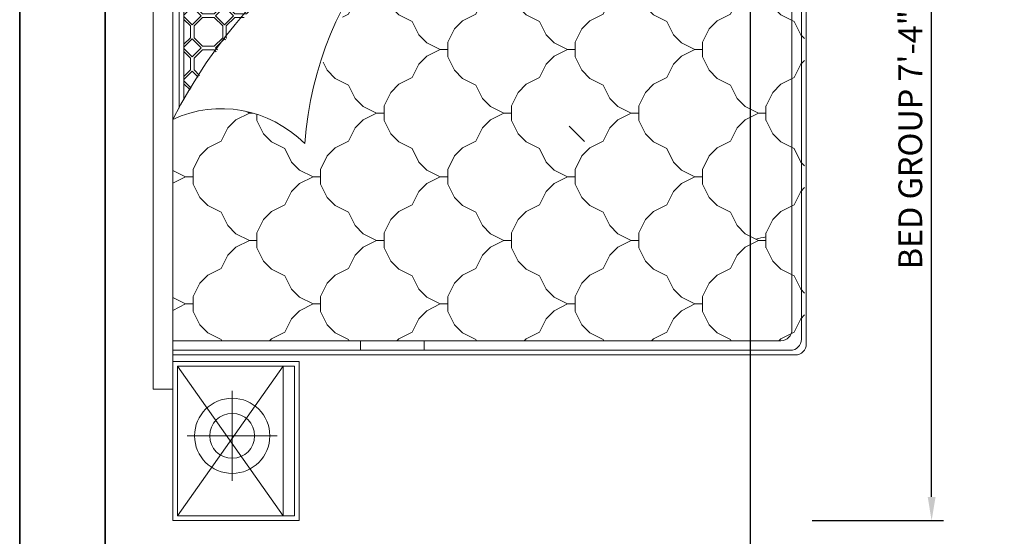
# Model space of a CAD drawing. Units: inches. Extents: x 1624 to 3956, y 1589 to 5028.
# Tile 12 of 16: x 1943 to 2046, y 2317 to 2372. Entities that reach past the tile are written whole.
import ezdxf

# ---------------------------------------------------------------- set-up
doc = ezdxf.new("R2010")
doc.units = ezdxf.units.IN
for name, color, linetype, lineweight in [('A-ANNO-DIMS', 2, 'Continuous', 13), ('A-FURN', 8, 'Continuous', 18), ('A-WALL', 7, 'Continuous', 35)]:
    doc.layers.add(name, color=color, linetype=linetype, lineweight=lineweight)
doc.styles.get("Standard").update_dxf_attribs({"font": 'arial.ttf'})
doc.dimstyles.new('Copy of ISO-25', dxfattribs={"dimtxt": 2.5, "dimasz": 2.5, "dimexe": 1.25, "dimexo": 0.625, "dimtad": 1, "dimdec": 1, "dimlunit": 4, "dimtxsty": 'Standard', "dimcen": 2.5, "dimadec": 0, "dimazin": 0, "dimtfac": 1, "dimtdec": 1, "dimtmove": 0, "dimatfit": 3, "dimfxl": 1, "dimarcsym": 0})

# ---------------------------------------------------------------- blocks, each defined once
blk = doc.blocks.new('A$C029D5C69')
for p, q in [((0.4164, 2.0693), (0.4164, 2.0066)), ((2.2315, 2.0693), (0.4164, 2.0693)), ((2.2315, 2.0066), (2.2315, 2.0693)), ((0, 1.606), (0, 2.0066)), ((0, 2.0066), (0.505, 2.0066)), ((0.4164, 2.0066), (2.2315, 2.0066)), ((0.505, 2.0066), (0.505, 1.606)), ((0.5252, 0.0351), (0.5252, 2.0066)), ((0.5403, 0.0502), (0.5403, 2.0066)), ((0.5706, 0.0805), (0.5706, 2.0066)), ((0.6869, 1.966), (0.6666, 2.0066)), ((0.7072, 2.0066), (0.6869, 1.966)), ((1.0902, 1.966), (1.0699, 2.0066)), ((1.1106, 2.0066), (1.0902, 1.966)), ((2.1114, 2.0087), (2.1114, 0.0351)), ((2.6479, 2.0066), (2.1429, 2.0066)), ((2.1429, 2.0066), (2.1429, 1.606)), ((2.6479, 1.606), (2.6479, 2.0066)), ((0.0151, 1.6211), (0.0151, 1.9915)), ((0.0151, 1.9915), (0.4899, 1.9915)), ((0.4899, 1.9915), (0.4899, 1.6211)), ((0.6869, 1.9425), (0.6869, 1.966)), ((0.6869, 1.9425), (0.6869, 1.966)), ((1.0902, 1.9425), (1.0902, 1.966)), ((1.0902, 1.9425), (1.0902, 1.966)), ((1.8954, 1.9865), (1.3081, 1.9865)), ((1.8954, 1.9713), (1.3339, 1.9713)), ((1.3849, 1.9713), (1.3656, 1.952)), ((1.3945, 1.9713), (1.3714, 1.9483)), ((1.4249, 1.945), (1.3986, 1.9713)), ((1.4288, 1.9507), (1.4081, 1.9713)), ((1.487, 1.9713), (1.4664, 1.9507)), ((1.4966, 1.9713), (1.4703, 1.945)), ((1.527, 1.945), (1.5007, 1.9713)), ((1.5309, 1.9507), (1.5102, 1.9713)), ((1.5891, 1.9713), (1.5685, 1.9507)), ((1.5987, 1.9713), (1.5724, 1.945)), ((1.6291, 1.945), (1.6028, 1.9713)), ((1.633, 1.9507), (1.6123, 1.9713)), ((1.6912, 1.9713), (1.6706, 1.9507)), ((1.7008, 1.9713), (1.6745, 1.945)), ((1.7312, 1.945), (1.7049, 1.9713)), ((1.7351, 1.9507), (1.7144, 1.9713)), ((1.7933, 1.9713), (1.7727, 1.9507)), ((1.8029, 1.9713), (1.7766, 1.945)), ((1.8333, 1.945), (1.807, 1.9713)), ((1.8372, 1.9507), (1.8165, 1.9713)), ((1.8954, 1.9713), (1.8748, 1.9507)), ((1.9043, 1.9707), (1.8787, 1.945)), ((1.9354, 1.945), (1.9114, 1.969)), ((2.6328, 1.9915), (2.158, 1.9915)), ((2.158, 1.9915), (2.158, 1.6211)), ((2.6328, 1.6211), (2.6328, 1.9915)), ((0.2689, 1.9609), (0.2689, 1.6764)), ((0.6634, 1.9425), (0.621, 1.9213)), ((0.6634, 1.9425), (0.621, 1.9213)), ((0.6869, 1.9425), (0.6634, 1.9425)), ((0.6869, 1.9425), (0.7104, 1.9425)), ((0.7528, 1.9213), (0.7104, 1.9425)), ((0.7528, 1.9213), (0.7104, 1.9425)), ((1.0668, 1.9425), (1.0244, 1.9213)), ((1.0668, 1.9425), (1.0244, 1.9213)), ((1.0902, 1.9425), (1.0668, 1.9425)), ((1.0902, 1.9425), (1.1137, 1.9425)), ((1.1561, 1.9213), (1.1137, 1.9425)), ((1.1561, 1.9213), (1.1137, 1.9425)), ((1.4249, 1.945), (1.4059, 1.926)), ((1.4288, 1.9394), (1.4116, 1.9222)), ((1.4476, 1.9507), (1.4288, 1.9507)), ((1.4288, 1.9393), (1.4476, 1.9393)), ((1.4476, 1.9507), (1.4664, 1.9507)), ((1.4664, 1.9393), (1.4476, 1.9393)), ((1.493, 1.9128), (1.4664, 1.9394)), ((1.4986, 1.9167), (1.4703, 1.945)), ((1.527, 1.945), (1.4986, 1.9167)), ((1.5309, 1.9394), (1.5043, 1.9128)), ((1.5497, 1.9507), (1.5309, 1.9507)), ((1.5309, 1.9393), (1.5497, 1.9393)), ((1.5497, 1.9507), (1.5685, 1.9507)), ((1.5685, 1.9393), (1.5497, 1.9393)), ((1.595, 1.9128), (1.5685, 1.9394)), ((1.6007, 1.9167), (1.5724, 1.945)), ((1.6291, 1.945), (1.6007, 1.9167)), ((1.633, 1.9394), (1.6064, 1.9128)), ((1.6518, 1.9507), (1.633, 1.9507)), ((1.633, 1.9393), (1.6518, 1.9393)), ((1.6518, 1.9507), (1.6706, 1.9507)), ((1.6706, 1.9393), (1.6518, 1.9393)), ((1.6971, 1.9128), (1.6706, 1.9394)), ((1.7028, 1.9167), (1.6745, 1.945)), ((1.7312, 1.945), (1.7028, 1.9167)), ((1.7351, 1.9394), (1.7085, 1.9128)), ((1.7539, 1.9507), (1.7351, 1.9507)), ((1.7351, 1.9393), (1.7539, 1.9393)), ((1.7539, 1.9507), (1.7727, 1.9507)), ((1.7727, 1.9393), (1.7539, 1.9393)), ((1.7992, 1.9128), (1.7727, 1.9394)), ((1.8049, 1.9167), (1.7766, 1.945)), ((1.8333, 1.945), (1.8049, 1.9167)), ((1.8372, 1.9394), (1.8106, 1.9128)), ((1.856, 1.9507), (1.8372, 1.9507)), ((1.8372, 1.9393), (1.856, 1.9393)), ((1.856, 1.9507), (1.8748, 1.9507)), ((1.8748, 1.9393), (1.856, 1.9393)), ((1.9013, 1.9128), (1.8748, 1.9394)), ((1.907, 1.9167), (1.8787, 1.945)), ((1.9354, 1.945), (1.907, 1.9167)), ((1.9393, 1.9394), (1.9127, 1.9128)), ((1.9393, 1.9393), (1.9404, 1.9393)), ((2.379, 1.9609), (2.379, 1.6764)), ((0.621, 1.9213), (0.5955, 1.8958)), ((0.7783, 1.8958), (0.7528, 1.9213)), ((1.0243, 1.9213), (0.9988, 1.8958)), ((1.1816, 1.8958), (1.1561, 1.9213)), ((1.493, 1.8752), (1.493, 1.9128)), ((1.5043, 1.8752), (1.5043, 1.9128)), ((1.595, 1.8752), (1.595, 1.9128)), ((1.6064, 1.8752), (1.6064, 1.9128)), ((1.6971, 1.8752), (1.6971, 1.9128)), ((1.7085, 1.8752), (1.7085, 1.9128)), ((1.7992, 1.8752), (1.7992, 1.9128)), ((1.8106, 1.8752), (1.8106, 1.9128)), ((1.9013, 1.8752), (1.9013, 1.9128)), ((1.9127, 1.8752), (1.9127, 1.9128)), ((1.9414, 1.688), (1.9414, 1.931)), ((1.9565, 1.688), (1.9565, 1.931)), ((0.5955, 1.8958), (0.5743, 1.8534)), ((0.7995, 1.8534), (0.7783, 1.8958)), ((0.9989, 1.8958), (0.9777, 1.8534)), ((1.2028, 1.8534), (1.1816, 1.8958)), ((1.493, 1.8752), (1.4867, 1.869)), ((1.5309, 1.8486), (1.5043, 1.8752)), ((1.595, 1.8752), (1.5685, 1.8486)), ((1.633, 1.8486), (1.6064, 1.8752)), ((1.6971, 1.8752), (1.6706, 1.8486)), ((1.7351, 1.8486), (1.7085, 1.8752)), ((1.7992, 1.8752), (1.7727, 1.8486)), ((1.8372, 1.8486), (1.8106, 1.8752)), ((1.9013, 1.8752), (1.8748, 1.8486)), ((1.9393, 1.8486), (1.9127, 1.8752)), ((0.5743, 1.8534), (0.5706, 1.8515)), ((0.5743, 1.8534), (0.5706, 1.8515)), ((0.8419, 1.8322), (0.7995, 1.8534)), ((0.8419, 1.8322), (0.7995, 1.8534)), ((0.9777, 1.8534), (0.9353, 1.8322)), ((0.9777, 1.8534), (0.9353, 1.8322)), ((1.2452, 1.8322), (1.2028, 1.8534)), ((1.2452, 1.8322), (1.2028, 1.8534)), ((1.4986, 1.8713), (1.4922, 1.8648)), ((1.527, 1.8429), (1.4986, 1.8713)), ((1.527, 1.8429), (1.5242, 1.8401)), ((1.5497, 1.8486), (1.5309, 1.8486)), ((1.5497, 1.8486), (1.5685, 1.8486)), ((1.6007, 1.8713), (1.5724, 1.8429)), ((1.6007, 1.8146), (1.5724, 1.8429)), ((1.6291, 1.8429), (1.6007, 1.8713)), ((1.6291, 1.8429), (1.6007, 1.8146)), ((1.6518, 1.8486), (1.633, 1.8486)), ((1.6518, 1.8486), (1.6706, 1.8486)), ((1.7028, 1.8713), (1.6745, 1.8429)), ((1.7028, 1.8146), (1.6745, 1.8429)), ((1.7312, 1.8429), (1.7028, 1.8713)), ((1.7312, 1.8429), (1.7028, 1.8146)), ((1.7539, 1.8486), (1.7351, 1.8486)), ((1.7539, 1.8486), (1.7727, 1.8486)), ((1.8049, 1.8713), (1.7766, 1.8429)), ((1.8049, 1.8146), (1.7766, 1.8429)), ((1.8333, 1.8429), (1.8049, 1.8713)), ((1.8333, 1.8429), (1.8049, 1.8146)), ((1.856, 1.8486), (1.8372, 1.8486)), ((1.856, 1.8486), (1.8748, 1.8486)), ((1.907, 1.8713), (1.8787, 1.8429)), ((1.907, 1.8146), (1.8787, 1.8429)), ((1.9354, 1.8429), (1.907, 1.8713)), ((1.9354, 1.8429), (1.907, 1.8146)), ((1.9414, 1.8486), (1.9393, 1.8486)), ((0.1267, 1.8186), (0.4111, 1.8186)), ((0.8674, 1.8067), (0.8419, 1.8322)), ((0.9352, 1.8322), (0.9097, 1.8067)), ((1.2707, 1.8067), (1.2452, 1.8322)), ((1.5309, 1.8373), (1.5295, 1.8359)), ((1.5309, 1.8373), (1.5497, 1.8373)), ((1.5685, 1.8373), (1.5497, 1.8373)), ((1.595, 1.8107), (1.5685, 1.8373)), ((1.595, 1.7806), (1.595, 1.8107)), ((1.633, 1.8373), (1.6064, 1.8107)), ((1.6064, 1.7731), (1.6064, 1.8107)), ((1.633, 1.8373), (1.6518, 1.8373)), ((1.6706, 1.8373), (1.6518, 1.8373)), ((1.6971, 1.8107), (1.6706, 1.8373)), ((1.6971, 1.7731), (1.6971, 1.8107)), ((1.7351, 1.8373), (1.7085, 1.8107)), ((1.7085, 1.7731), (1.7085, 1.8107)), ((1.7351, 1.8373), (1.7539, 1.8373)), ((1.7727, 1.8373), (1.7539, 1.8373)), ((1.7992, 1.8107), (1.7727, 1.8373)), ((1.7992, 1.7731), (1.7992, 1.8107)), ((1.8372, 1.8373), (1.8106, 1.8107)), ((1.8106, 1.7731), (1.8106, 1.8107)), ((1.8372, 1.8373), (1.856, 1.8373)), ((1.8748, 1.8373), (1.856, 1.8373)), ((1.9013, 1.8107), (1.8748, 1.8373)), ((1.9013, 1.7731), (1.9013, 1.8107)), ((1.9393, 1.8373), (1.9127, 1.8107)), ((1.9127, 1.7731), (1.9127, 1.8107)), ((1.9393, 1.8373), (1.9414, 1.8373)), ((2.2367, 1.8186), (2.5212, 1.8186)), ((0.8886, 1.7643), (0.8674, 1.8067)), ((0.9098, 1.8067), (0.8886, 1.7643)), ((1.2919, 1.7643), (1.2707, 1.8067)), ((0.8886, 1.7408), (0.8886, 1.7643)), ((1.2981, 1.7768), (1.2919, 1.7643)), ((1.2919, 1.7519), (1.2919, 1.7643)), ((1.633, 1.7465), (1.6064, 1.7731)), ((1.6971, 1.7731), (1.6706, 1.7465)), ((1.7028, 1.7692), (1.6745, 1.7408)), ((1.7312, 1.7408), (1.7028, 1.7692)), ((1.7351, 1.7465), (1.7085, 1.7731)), ((1.7992, 1.7731), (1.7727, 1.7465)), ((1.8049, 1.7692), (1.7766, 1.7408)), ((1.8333, 1.7408), (1.8049, 1.7692)), ((1.8372, 1.7465), (1.8106, 1.7731)), ((1.9013, 1.7731), (1.8748, 1.7465)), ((1.907, 1.7692), (1.8787, 1.7408)), ((1.9354, 1.7408), (1.907, 1.7692)), ((1.9393, 1.7465), (1.9127, 1.7731)), ((0.8227, 1.7196), (0.7972, 1.6941)), ((0.8651, 1.7408), (0.8227, 1.7196)), ((0.8651, 1.7408), (0.8227, 1.7196)), ((0.912, 1.7408), (0.8651, 1.7408)), ((0.9544, 1.7196), (0.912, 1.7408)), ((0.9544, 1.7196), (0.912, 1.7408)), ((0.98, 1.6941), (0.9545, 1.7196)), ((1.226, 1.7196), (1.2005, 1.6941)), ((1.2684, 1.7408), (1.226, 1.7196)), ((1.2684, 1.7408), (1.226, 1.7196)), ((1.2885, 1.7408), (1.2684, 1.7408)), ((1.6518, 1.7465), (1.633, 1.7465)), ((1.6443, 1.7352), (1.6518, 1.7352)), ((1.6518, 1.7465), (1.6706, 1.7465)), ((1.6706, 1.7352), (1.6518, 1.7352)), ((1.6971, 1.7086), (1.6706, 1.7352)), ((1.7028, 1.7125), (1.6745, 1.7408)), ((1.7312, 1.7408), (1.7028, 1.7125)), ((1.7351, 1.7352), (1.7085, 1.7086)), ((1.7539, 1.7465), (1.7351, 1.7465)), ((1.7351, 1.7352), (1.7539, 1.7352)), ((1.7539, 1.7465), (1.7727, 1.7465)), ((1.7727, 1.7352), (1.7539, 1.7352)), ((1.7992, 1.7086), (1.7727, 1.7352)), ((1.8049, 1.7125), (1.7766, 1.7408)), ((1.8333, 1.7408), (1.8049, 1.7125)), ((1.8372, 1.7352), (1.8106, 1.7086)), ((1.856, 1.7465), (1.8372, 1.7465)), ((1.8372, 1.7352), (1.856, 1.7352)), ((1.856, 1.7465), (1.8748, 1.7465)), ((1.8748, 1.7352), (1.856, 1.7352)), ((1.9013, 1.7086), (1.8748, 1.7352)), ((1.907, 1.7125), (1.8787, 1.7408)), ((1.9354, 1.7408), (1.907, 1.7125)), ((1.9393, 1.7352), (1.9127, 1.7086)), ((1.9414, 1.7465), (1.9393, 1.7465)), ((1.9393, 1.7352), (1.9414, 1.7352)), ((0.5766, 1.6941), (0.5706, 1.7002)), ((0.5978, 1.6517), (0.5766, 1.6941)), ((0.7972, 1.6941), (0.776, 1.6517)), ((1.0011, 1.6517), (0.9799, 1.6941)), ((1.2005, 1.6941), (1.1793, 1.6517)), ((1.6971, 1.682), (1.6971, 1.7086)), ((1.7085, 1.671), (1.7085, 1.7086)), ((1.7992, 1.671), (1.7992, 1.7086)), ((1.8106, 1.671), (1.8106, 1.7086)), ((1.9013, 1.671), (1.9013, 1.7086)), ((1.9127, 1.671), (1.9127, 1.7086)), ((2.5551, 1.6275), (2.5551, 1.696)), ((1.7318, 1.6477), (1.7085, 1.671)), ((1.7992, 1.671), (1.7759, 1.6477)), ((1.8049, 1.6671), (1.7855, 1.6477)), ((1.8244, 1.6477), (1.8049, 1.6671)), ((1.8339, 1.6477), (1.8106, 1.671)), ((1.9013, 1.671), (1.878, 1.6477)), ((1.907, 1.6671), (1.8876, 1.6477)), ((1.9202, 1.6539), (1.907, 1.6671)), ((1.926, 1.6577), (1.9127, 1.671)), ((0.6402, 1.6305), (0.5978, 1.6517)), ((0.6402, 1.6305), (0.5978, 1.6517)), ((0.6657, 1.605), (0.6402, 1.6305)), ((0.7336, 1.6305), (0.7081, 1.605)), ((0.776, 1.6517), (0.7336, 1.6305)), ((0.776, 1.6517), (0.7336, 1.6305)), ((1.0435, 1.6305), (1.0011, 1.6517)), ((1.0435, 1.6305), (1.0011, 1.6517)), ((1.0691, 1.605), (1.0436, 1.6305)), ((1.1369, 1.6305), (1.1114, 1.605)), ((1.1793, 1.6517), (1.1369, 1.6305)), ((1.1793, 1.6517), (1.1369, 1.6305)), ((1.8961, 1.6477), (1.7289, 1.6477)), ((1.8961, 1.6325), (1.7422, 1.6325)), ((0.505, 1.606), (0, 1.606)), ((0.4899, 1.6211), (0.0151, 1.6211)), ((0.6869, 1.5626), (0.6657, 1.605)), ((0.7081, 1.605), (0.6869, 1.5626)), ((1.0902, 1.5626), (1.069, 1.605)), ((1.1114, 1.605), (1.0902, 1.5626)), ((2.1429, 1.606), (2.6479, 1.606)), ((2.158, 1.6211), (2.6328, 1.6211)), ((0.6869, 1.5392), (0.6869, 1.5626)), ((0.6869, 1.5392), (0.6869, 1.5626)), ((1.0902, 1.5392), (1.0902, 1.5626)), ((1.0902, 1.5392), (1.0902, 1.5626)), ((0.6634, 1.5391), (0.621, 1.5179)), ((0.6634, 1.5391), (0.621, 1.5179)), ((0.6869, 1.5392), (0.6634, 1.5392)), ((0.6869, 1.5392), (0.7104, 1.5392)), ((0.7528, 1.5179), (0.7104, 1.5391)), ((0.7528, 1.5179), (0.7104, 1.5391)), ((1.0668, 1.5391), (1.0244, 1.5179)), ((1.0668, 1.5391), (1.0244, 1.5179)), ((1.0902, 1.5392), (1.0668, 1.5392)), ((1.0902, 1.5392), (1.1137, 1.5392)), ((1.1561, 1.5179), (1.1137, 1.5391)), ((1.1561, 1.5179), (1.1137, 1.5391)), ((1.4534, 1.5308), (1.4277, 1.5179)), ((1.4534, 1.5308), (1.4277, 1.5179)), ((0.621, 1.5179), (0.5955, 1.4924)), ((0.7783, 1.4924), (0.7528, 1.5179)), ((1.0243, 1.5179), (0.9988, 1.4924)), ((1.1816, 1.4924), (1.1561, 1.5179)), ((1.4277, 1.5179), (1.4022, 1.4924)), ((0.5955, 1.4925), (0.5743, 1.4501)), ((0.7995, 1.4501), (0.7783, 1.4925)), ((0.9989, 1.4925), (0.9777, 1.4501)), ((1.2028, 1.4501), (1.1816, 1.4925)), ((1.4022, 1.4925), (1.381, 1.4501)), ((1.6062, 1.4501), (1.5966, 1.4692)), ((0.5743, 1.45), (0.5706, 1.4481)), ((0.5743, 1.45), (0.5706, 1.4481)), ((0.8419, 1.4288), (0.7995, 1.45)), ((0.8419, 1.4288), (0.7995, 1.45)), ((0.9777, 1.45), (0.9353, 1.4288)), ((0.9777, 1.45), (0.9353, 1.4288)), ((1.2452, 1.4288), (1.2028, 1.45)), ((1.2452, 1.4288), (1.2028, 1.45)), ((1.381, 1.45), (1.3386, 1.4288)), ((1.381, 1.45), (1.3386, 1.4288)), ((1.6486, 1.4288), (1.6062, 1.45)), ((1.6486, 1.4288), (1.6062, 1.45)), ((0.5403, 1.4117), (0.5706, 1.4117)), ((0.8674, 1.4033), (0.8419, 1.4288)), ((0.9352, 1.4288), (0.9097, 1.4033)), ((1.2707, 1.4033), (1.2452, 1.4288)), ((1.3386, 1.4288), (1.3131, 1.4033)), ((1.6741, 1.4033), (1.6486, 1.4288)), ((0.8886, 1.361), (0.8674, 1.4034)), ((0.9098, 1.4034), (0.8886, 1.361)), ((1.2919, 1.361), (1.2707, 1.4034)), ((1.3131, 1.4034), (1.2919, 1.361)), ((1.6953, 1.361), (1.6741, 1.4034)), ((1.714, 1.3984), (1.6953, 1.361)), ((0.8886, 1.3375), (0.8886, 1.3609)), ((1.2919, 1.3375), (1.2919, 1.3609)), ((1.6953, 1.3375), (1.6953, 1.3609)), ((0.8227, 1.3163), (0.7972, 1.2908)), ((0.8651, 1.3374), (0.8227, 1.3162)), ((0.8651, 1.3374), (0.8227, 1.3162)), ((0.912, 1.3375), (0.8651, 1.3375)), ((0.9544, 1.3162), (0.912, 1.3374)), ((0.9544, 1.3162), (0.912, 1.3374)), ((0.98, 1.2908), (0.9545, 1.3163)), ((1.226, 1.3163), (1.2005, 1.2908)), ((1.2684, 1.3374), (1.226, 1.3162)), ((1.2684, 1.3374), (1.226, 1.3162)), ((1.3154, 1.3375), (1.2684, 1.3375)), ((1.3578, 1.3162), (1.3154, 1.3374)), ((1.3578, 1.3162), (1.3154, 1.3374)), ((1.3833, 1.2908), (1.3578, 1.3163)), ((1.6294, 1.3163), (1.6039, 1.2908)), ((1.6718, 1.3374), (1.6294, 1.3162)), ((1.6718, 1.3374), (1.6294, 1.3162)), ((1.7187, 1.3375), (1.6718, 1.3375)), ((1.7611, 1.3162), (1.7187, 1.3374)), ((1.7611, 1.3162), (1.7187, 1.3374)), ((1.7867, 1.2908), (1.7611, 1.3163)), ((0.5766, 1.2908), (0.5706, 1.2968)), ((0.5978, 1.2484), (0.5766, 1.2908)), ((0.7972, 1.2908), (0.776, 1.2484)), ((1.0011, 1.2484), (0.9799, 1.2908)), ((1.2005, 1.2908), (1.1793, 1.2484)), ((1.4045, 1.2484), (1.3833, 1.2908)), ((1.6039, 1.2908), (1.5827, 1.2484)), ((1.8078, 1.2484), (1.7866, 1.2908)), ((0.6402, 1.2271), (0.5978, 1.2483)), ((0.6402, 1.2271), (0.5978, 1.2483)), ((0.776, 1.2483), (0.7336, 1.2271)), ((0.776, 1.2483), (0.7336, 1.2271)), ((1.0435, 1.2271), (1.0011, 1.2483)), ((1.0435, 1.2271), (1.0011, 1.2483)), ((1.1793, 1.2483), (1.1369, 1.2271)), ((1.1793, 1.2483), (1.1369, 1.2271)), ((1.4469, 1.2271), (1.4045, 1.2483)), ((1.4469, 1.2271), (1.4045, 1.2483)), ((1.5827, 1.2483), (1.5403, 1.2271)), ((1.5827, 1.2483), (1.5403, 1.2271)), ((1.8502, 1.2271), (1.8078, 1.2483)), ((1.8502, 1.2271), (1.8078, 1.2483)), ((0.6657, 1.2017), (0.6402, 1.2272)), ((0.7336, 1.2272), (0.7081, 1.2017)), ((1.0691, 1.2017), (1.0436, 1.2272)), ((1.1369, 1.2272), (1.1114, 1.2017)), ((1.4724, 1.2017), (1.4469, 1.2272)), ((1.5403, 1.2272), (1.5148, 1.2017)), ((1.8758, 1.2017), (1.8503, 1.2272)), ((0.5403, 1.21), (0.5706, 1.21)), ((0.6869, 1.1593), (0.6657, 1.2017)), ((0.7081, 1.2017), (0.6869, 1.1593)), ((1.0902, 1.1593), (1.069, 1.2017)), ((1.1114, 1.2017), (1.0902, 1.1593)), ((1.4936, 1.1593), (1.4724, 1.2017)), ((1.5148, 1.2017), (1.4936, 1.1593)), ((1.8969, 1.1593), (1.8757, 1.2017)), ((1.9181, 1.2017), (1.8969, 1.1593)), ((1.9215, 1.2051), (1.9181, 1.2017)), ((0.6869, 1.1358), (0.6869, 1.1593)), ((0.6869, 1.1358), (0.6869, 1.1593)), ((1.0902, 1.1358), (1.0902, 1.1593)), ((1.0902, 1.1358), (1.0902, 1.1593)), ((1.4936, 1.1358), (1.4936, 1.1593)), ((1.4936, 1.1358), (1.4936, 1.1593)), ((1.8969, 1.1358), (1.8969, 1.1593)), ((1.8969, 1.1358), (1.8969, 1.1593)), ((0.6634, 1.1358), (0.621, 1.1146)), ((0.6634, 1.1358), (0.621, 1.1146)), ((0.6869, 1.1358), (0.6634, 1.1358)), ((0.6869, 1.1358), (0.7104, 1.1358)), ((0.7528, 1.1146), (0.7104, 1.1358)), ((0.7528, 1.1146), (0.7104, 1.1358)), ((1.0668, 1.1358), (1.0244, 1.1146)), ((1.0668, 1.1358), (1.0244, 1.1146)), ((1.0902, 1.1358), (1.0668, 1.1358)), ((1.0902, 1.1358), (1.1137, 1.1358)), ((1.1561, 1.1146), (1.1137, 1.1358)), ((1.1561, 1.1146), (1.1137, 1.1358)), ((1.4701, 1.1358), (1.4277, 1.1146)), ((1.4701, 1.1358), (1.4277, 1.1146)), ((1.4936, 1.1358), (1.4701, 1.1358)), ((1.4936, 1.1358), (1.5171, 1.1358)), ((1.5595, 1.1146), (1.5171, 1.1358)), ((1.5595, 1.1146), (1.5171, 1.1358)), ((1.8735, 1.1358), (1.8311, 1.1146)), ((1.8735, 1.1358), (1.8311, 1.1146)), ((1.8969, 1.1358), (1.8735, 1.1358)), ((1.8969, 1.1358), (1.9204, 1.1358)), ((1.9628, 1.1146), (1.9204, 1.1358)), ((1.9628, 1.1146), (1.9204, 1.1358)), ((0.621, 1.1146), (0.5955, 1.0891)), ((0.7783, 1.0891), (0.7528, 1.1146)), ((1.0243, 1.1146), (0.9988, 1.0891)), ((1.1816, 1.0891), (1.1561, 1.1146)), ((1.4277, 1.1146), (1.4022, 1.0891)), ((1.585, 1.0891), (1.5595, 1.1146)), ((1.831, 1.1146), (1.8055, 1.0891)), ((1.9883, 1.0891), (1.9628, 1.1146)), ((0.5955, 1.0891), (0.5743, 1.0467)), ((0.7995, 1.0467), (0.7783, 1.0891)), ((0.9989, 1.0891), (0.9777, 1.0467)), ((1.2028, 1.0467), (1.1816, 1.0891)), ((1.4022, 1.0891), (1.381, 1.0467)), ((1.6062, 1.0467), (1.585, 1.0891)), ((1.8056, 1.0891), (1.7844, 1.0467)), ((2.0095, 1.0467), (1.9883, 1.0891)), ((0.5743, 1.0467), (0.5706, 1.0448)), ((0.5743, 1.0467), (0.5706, 1.0448)), ((0.8419, 1.0255), (0.7995, 1.0467)), ((0.8419, 1.0255), (0.7995, 1.0467)), ((0.9777, 1.0467), (0.9353, 1.0255)), ((0.9777, 1.0467), (0.9353, 1.0255)), ((1.2452, 1.0255), (1.2028, 1.0467)), ((1.2452, 1.0255), (1.2028, 1.0467)), ((1.381, 1.0467), (1.3386, 1.0255)), ((1.381, 1.0467), (1.3386, 1.0255)), ((1.6486, 1.0255), (1.6062, 1.0467)), ((1.6486, 1.0255), (1.6062, 1.0467)), ((1.7844, 1.0467), (1.742, 1.0255)), ((1.7844, 1.0467), (1.742, 1.0255)), ((2.0276, 1.0376), (2.0095, 1.0467)), ((2.0276, 1.0376), (2.0095, 1.0467)), ((0.8674, 1), (0.8419, 1.0255)), ((0.8886, 0.9576), (0.8674, 1)), ((0.9098, 1), (0.8886, 0.9576)), ((0.9352, 1.0255), (0.9097, 1)), ((1.2707, 1), (1.2452, 1.0255)), ((1.2919, 0.9576), (1.2707, 1)), ((1.3131, 1), (1.2919, 0.9576)), ((1.3386, 1.0255), (1.3131, 1)), ((1.6741, 1), (1.6486, 1.0255)), ((1.6953, 0.9576), (1.6741, 1)), ((1.7165, 1), (1.6953, 0.9576)), ((1.7419, 1.0255), (1.7164, 1)), ((0.8886, 0.9341), (0.8886, 0.9576)), ((1.2919, 0.9341), (1.2919, 0.9576)), ((1.6953, 0.9341), (1.6953, 0.9576)), ((2.066, 0.9457), (2.066, 0.0805)), ((0.8227, 0.9129), (0.7972, 0.8874)), ((0.8651, 0.9341), (0.8227, 0.9129)), ((0.8651, 0.9341), (0.8227, 0.9129)), ((0.912, 0.9341), (0.8651, 0.9341)), ((0.9544, 0.9129), (0.912, 0.9341)), ((0.9544, 0.9129), (0.912, 0.9341)), ((0.98, 0.8874), (0.9545, 0.9129)), ((1.226, 0.9129), (1.2005, 0.8874)), ((1.2684, 0.9341), (1.226, 0.9129)), ((1.2684, 0.9341), (1.226, 0.9129)), ((1.3154, 0.9341), (1.2684, 0.9341)), ((1.3578, 0.9129), (1.3154, 0.9341)), ((1.3578, 0.9129), (1.3154, 0.9341)), ((1.3833, 0.8874), (1.3578, 0.9129)), ((1.6294, 0.9129), (1.6039, 0.8874)), ((1.6718, 0.9341), (1.6294, 0.9129)), ((1.6718, 0.9341), (1.6294, 0.9129)), ((1.7187, 0.9341), (1.6718, 0.9341)), ((1.7611, 0.9129), (1.7187, 0.9341)), ((1.7611, 0.9129), (1.7187, 0.9341)), ((1.7867, 0.8874), (1.7611, 0.9129)), ((2.0327, 0.9129), (2.0072, 0.8874)), ((2.066, 0.9295), (2.0327, 0.9129)), ((2.066, 0.9295), (2.0327, 0.9129)), ((0.5766, 0.8874), (0.5706, 0.8935)), ((0.5978, 0.845), (0.5766, 0.8874)), ((0.7972, 0.8874), (0.776, 0.845)), ((1.0011, 0.845), (0.9799, 0.8874)), ((1.2005, 0.8874), (1.1793, 0.845)), ((1.4045, 0.845), (1.3833, 0.8874)), ((1.6039, 0.8874), (1.5827, 0.845)), ((1.8078, 0.845), (1.7866, 0.8874)), ((2.0072, 0.8874), (1.986, 0.845)), ((0.6402, 0.8238), (0.5978, 0.845)), ((0.6402, 0.8238), (0.5978, 0.845)), ((0.776, 0.845), (0.7336, 0.8238)), ((0.776, 0.845), (0.7336, 0.8238)), ((1.0435, 0.8238), (1.0011, 0.845)), ((1.0435, 0.8238), (1.0011, 0.845)), ((1.1793, 0.845), (1.1369, 0.8238)), ((1.1793, 0.845), (1.1369, 0.8238)), ((1.4469, 0.8238), (1.4045, 0.845)), ((1.4469, 0.8238), (1.4045, 0.845)), ((1.5827, 0.845), (1.5403, 0.8238)), ((1.5827, 0.845), (1.5403, 0.8238)), ((1.8502, 0.8238), (1.8078, 0.845)), ((1.8502, 0.8238), (1.8078, 0.845)), ((1.986, 0.845), (1.9436, 0.8238)), ((1.986, 0.845), (1.9436, 0.8238)), ((0.6657, 0.7983), (0.6402, 0.8238)), ((0.7336, 0.8238), (0.7081, 0.7983)), ((1.0691, 0.7983), (1.0436, 0.8238)), ((1.1369, 0.8238), (1.1114, 0.7983)), ((1.4724, 0.7983), (1.4469, 0.8238)), ((1.5403, 0.8238), (1.5148, 0.7983)), ((1.8758, 0.7983), (1.8503, 0.8238)), ((1.9436, 0.8238), (1.9181, 0.7983)), ((2.0962, 0.8369), (2.0962, 0.0502)), ((0.6869, 0.7559), (0.6657, 0.7983)), ((0.7081, 0.7983), (0.6869, 0.7559)), ((1.0902, 0.7559), (1.069, 0.7983)), ((1.1114, 0.7983), (1.0902, 0.7559)), ((1.4936, 0.7559), (1.4724, 0.7983)), ((1.5148, 0.7983), (1.4936, 0.7559)), ((1.8969, 0.7559), (1.8757, 0.7983)), ((1.9181, 0.7983), (1.8969, 0.7559)), ((0.6869, 0.7325), (0.6869, 0.7559)), ((0.6869, 0.7325), (0.6869, 0.7559)), ((1.0902, 0.7325), (1.0902, 0.7559)), ((1.0902, 0.7325), (1.0902, 0.7559)), ((1.2024, 0.7028), (1.2503, 0.7507)), ((1.4936, 0.7325), (1.4936, 0.7559)), ((1.4936, 0.7325), (1.4936, 0.7559)), ((1.8969, 0.7325), (1.8969, 0.7559)), ((1.8969, 0.7325), (1.8969, 0.7559)), ((0.6634, 0.7324), (0.621, 0.7112)), ((0.6634, 0.7324), (0.621, 0.7112)), ((0.6869, 0.7325), (0.6634, 0.7325)), ((0.6869, 0.7325), (0.7104, 0.7325)), ((0.7528, 0.7112), (0.7104, 0.7324)), ((0.7528, 0.7112), (0.7104, 0.7324)), ((1.0668, 0.7324), (1.0244, 0.7112)), ((1.0668, 0.7324), (1.0244, 0.7112)), ((1.0902, 0.7325), (1.0668, 0.7325)), ((1.0902, 0.7325), (1.1137, 0.7325)), ((1.1561, 0.7112), (1.1137, 0.7324)), ((1.1561, 0.7112), (1.1137, 0.7324)), ((1.4701, 0.7324), (1.4277, 0.7112)), ((1.4701, 0.7324), (1.4277, 0.7112)), ((1.4936, 0.7325), (1.4701, 0.7325)), ((1.4936, 0.7325), (1.5171, 0.7325)), ((1.5595, 0.7112), (1.5171, 0.7324)), ((1.5595, 0.7112), (1.5171, 0.7324)), ((1.8735, 0.7324), (1.8311, 0.7112)), ((1.8735, 0.7324), (1.8311, 0.7112)), ((1.8969, 0.7325), (1.8735, 0.7325)), ((1.8969, 0.7325), (1.9204, 0.7325)), ((1.9628, 0.7112), (1.9204, 0.7324)), ((1.9628, 0.7112), (1.9204, 0.7324)), ((0.621, 0.7113), (0.5955, 0.6858)), ((0.7783, 0.6858), (0.7528, 0.7113)), ((1.0243, 0.7113), (0.9988, 0.6858)), ((1.1816, 0.6858), (1.1561, 0.7113)), ((1.4277, 0.7113), (1.4022, 0.6858)), ((1.585, 0.6858), (1.5595, 0.7113)), ((1.831, 0.7113), (1.8055, 0.6858)), ((1.9883, 0.6858), (1.9628, 0.7113)), ((0.5955, 0.6858), (0.5743, 0.6434)), ((0.7995, 0.6434), (0.7783, 0.6858)), ((0.9989, 0.6858), (0.9777, 0.6434)), ((1.2028, 0.6434), (1.1816, 0.6858)), ((1.4022, 0.6858), (1.381, 0.6434)), ((1.6062, 0.6434), (1.585, 0.6858)), ((1.8056, 0.6858), (1.7844, 0.6434)), ((2.0095, 0.6434), (1.9883, 0.6858)), ((0.5743, 0.6433), (0.5706, 0.6414)), ((0.5743, 0.6433), (0.5706, 0.6414)), ((0.8419, 0.6221), (0.7995, 0.6433)), ((0.8419, 0.6221), (0.7995, 0.6433)), ((0.9777, 0.6433), (0.9353, 0.6221)), ((0.9777, 0.6433), (0.9353, 0.6221)), ((1.2452, 0.6221), (1.2028, 0.6433)), ((1.2452, 0.6221), (1.2028, 0.6433)), ((1.381, 0.6433), (1.3386, 0.6221)), ((1.381, 0.6433), (1.3386, 0.6221)), ((1.6486, 0.6221), (1.6062, 0.6433)), ((1.6486, 0.6221), (1.6062, 0.6433)), ((1.7844, 0.6433), (1.742, 0.6221)), ((1.7844, 0.6433), (1.742, 0.6221)), ((2.0519, 0.6221), (2.0095, 0.6433)), ((2.0519, 0.6221), (2.0095, 0.6433)), ((0.8674, 0.5967), (0.8419, 0.6222)), ((0.8886, 0.5543), (0.8674, 0.5967)), ((0.9098, 0.5967), (0.8886, 0.5543)), ((0.9352, 0.6222), (0.9097, 0.5967)), ((1.2707, 0.5967), (1.2452, 0.6222)), ((1.2919, 0.5543), (1.2707, 0.5967)), ((1.3131, 0.5967), (1.2919, 0.5543)), ((1.3386, 0.6222), (1.3131, 0.5967)), ((1.6741, 0.5967), (1.6486, 0.6222)), ((1.6953, 0.5543), (1.6741, 0.5967)), ((1.7165, 0.5967), (1.6953, 0.5543)), ((1.7419, 0.6222), (1.7164, 0.5967)), ((2.066, 0.6081), (2.0519, 0.6222)), ((0.8651, 0.5308), (0.8227, 0.5096)), ((0.8651, 0.5308), (0.8227, 0.5096)), ((0.912, 0.5308), (0.8651, 0.5308)), ((0.8886, 0.5308), (0.8886, 0.5543)), ((0.9544, 0.5096), (0.912, 0.5308)), ((0.9544, 0.5096), (0.912, 0.5308)), ((1.2684, 0.5308), (1.226, 0.5096)), ((1.2684, 0.5308), (1.226, 0.5096)), ((1.3154, 0.5308), (1.2684, 0.5308)), ((1.2919, 0.5308), (1.2919, 0.5543)), ((1.3578, 0.5096), (1.3154, 0.5308)), ((1.3578, 0.5096), (1.3154, 0.5308)), ((1.6718, 0.5308), (1.6294, 0.5096)), ((1.6718, 0.5308), (1.6294, 0.5096)), ((1.7187, 0.5308), (1.6718, 0.5308)), ((1.6953, 0.5308), (1.6953, 0.5543)), ((1.7611, 0.5096), (1.7187, 0.5308)), ((1.7611, 0.5096), (1.7187, 0.5308)), ((0.8227, 0.5096), (0.7972, 0.4841)), ((0.98, 0.4841), (0.9545, 0.5096)), ((1.226, 0.5096), (1.2005, 0.4841)), ((1.3833, 0.4841), (1.3578, 0.5096)), ((1.6294, 0.5096), (1.6039, 0.4841)), ((1.7867, 0.4841), (1.7611, 0.5096)), ((2.0327, 0.5096), (2.0072, 0.4841)), ((2.066, 0.5262), (2.0327, 0.5096)), ((2.066, 0.5262), (2.0327, 0.5096)), ((0.5766, 0.4841), (0.5706, 0.4901)), ((0.5978, 0.4417), (0.5766, 0.4841)), ((0.7972, 0.4841), (0.776, 0.4417)), ((1.0011, 0.4417), (0.9799, 0.4841)), ((1.2005, 0.4841), (1.1793, 0.4417)), ((1.4045, 0.4417), (1.3833, 0.4841)), ((1.6039, 0.4841), (1.5827, 0.4417)), ((1.8078, 0.4417), (1.7866, 0.4841)), ((2.0072, 0.4841), (1.986, 0.4417)), ((0.6402, 0.4205), (0.5978, 0.4417)), ((0.6402, 0.4205), (0.5978, 0.4417)), ((0.776, 0.4417), (0.7336, 0.4205)), ((0.776, 0.4417), (0.7336, 0.4205)), ((1.0435, 0.4205), (1.0011, 0.4417)), ((1.0435, 0.4205), (1.0011, 0.4417)), ((1.1793, 0.4417), (1.1369, 0.4205)), ((1.1793, 0.4417), (1.1369, 0.4205)), ((1.4469, 0.4205), (1.4045, 0.4417)), ((1.4469, 0.4205), (1.4045, 0.4417)), ((1.5827, 0.4417), (1.5403, 0.4205)), ((1.5827, 0.4417), (1.5403, 0.4205)), ((1.8502, 0.4205), (1.8078, 0.4417)), ((1.8502, 0.4205), (1.8078, 0.4417)), ((1.986, 0.4417), (1.9436, 0.4205)), ((1.986, 0.4417), (1.9436, 0.4205)), ((0.6657, 0.395), (0.6402, 0.4205)), ((0.7336, 0.4205), (0.7081, 0.395)), ((1.0691, 0.395), (1.0436, 0.4205)), ((1.1369, 0.4205), (1.1114, 0.395)), ((1.4724, 0.395), (1.4469, 0.4205)), ((1.5403, 0.4205), (1.5148, 0.395)), ((1.8758, 0.395), (1.8503, 0.4205)), ((1.9436, 0.4205), (1.9181, 0.395)), ((0.6869, 0.3526), (0.6657, 0.395)), ((0.7081, 0.395), (0.6869, 0.3526)), ((1.0902, 0.3526), (1.069, 0.395)), ((1.1114, 0.395), (1.0902, 0.3526)), ((1.4936, 0.3526), (1.4724, 0.395)), ((1.5148, 0.395), (1.4936, 0.3526)), ((1.8969, 0.3526), (1.8757, 0.395)), ((1.9181, 0.395), (1.8969, 0.3526)), ((0.6869, 0.3291), (0.6869, 0.3526)), ((0.6869, 0.3291), (0.6869, 0.3526)), ((1.0902, 0.3291), (1.0902, 0.3526)), ((1.0902, 0.3291), (1.0902, 0.3526)), ((1.4936, 0.3291), (1.4936, 0.3526)), ((1.4936, 0.3291), (1.4936, 0.3526)), ((1.8969, 0.3291), (1.8969, 0.3526)), ((1.8969, 0.3291), (1.8969, 0.3526)), ((0.6634, 0.3291), (0.621, 0.3079)), ((0.6634, 0.3291), (0.621, 0.3079)), ((0.6869, 0.3291), (0.6634, 0.3291)), ((0.6869, 0.3291), (0.7104, 0.3291)), ((0.7528, 0.3079), (0.7104, 0.3291)), ((0.7528, 0.3079), (0.7104, 0.3291)), ((1.0668, 0.3291), (1.0244, 0.3079)), ((1.0668, 0.3291), (1.0244, 0.3079)), ((1.0902, 0.3291), (1.0668, 0.3291)), ((1.0902, 0.3291), (1.1137, 0.3291)), ((1.1561, 0.3079), (1.1137, 0.3291)), ((1.1561, 0.3079), (1.1137, 0.3291)), ((1.4701, 0.3291), (1.4277, 0.3079)), ((1.4701, 0.3291), (1.4277, 0.3079)), ((1.4936, 0.3291), (1.4701, 0.3291)), ((1.4936, 0.3291), (1.5171, 0.3291)), ((1.5595, 0.3079), (1.5171, 0.3291)), ((1.5595, 0.3079), (1.5171, 0.3291)), ((1.8735, 0.3291), (1.8311, 0.3079)), ((1.8735, 0.3291), (1.8311, 0.3079)), ((1.8969, 0.3291), (1.8735, 0.3291)), ((1.8969, 0.3291), (1.9204, 0.3291)), ((1.9628, 0.3079), (1.9204, 0.3291)), ((1.9628, 0.3079), (1.9204, 0.3291)), ((0.5955, 0.2824), (0.5743, 0.24)), ((0.621, 0.3079), (0.5955, 0.2824)), ((0.7783, 0.2824), (0.7528, 0.3079)), ((0.7995, 0.24), (0.7783, 0.2824)), ((0.9989, 0.2824), (0.9777, 0.24)), ((1.0243, 0.3079), (0.9988, 0.2824)), ((1.1816, 0.2824), (1.1561, 0.3079)), ((1.2028, 0.24), (1.1816, 0.2824)), ((1.4022, 0.2824), (1.381, 0.24)), ((1.4277, 0.3079), (1.4022, 0.2824)), ((1.585, 0.2824), (1.5595, 0.3079)), ((1.6062, 0.24), (1.585, 0.2824)), ((1.8056, 0.2824), (1.7844, 0.24)), ((1.831, 0.3079), (1.8055, 0.2824)), ((1.9883, 0.2824), (1.9628, 0.3079)), ((2.0095, 0.24), (1.9883, 0.2824)), ((0.5743, 0.24), (0.5706, 0.2381)), ((0.5743, 0.24), (0.5706, 0.2381)), ((0.8419, 0.2188), (0.7995, 0.24)), ((0.8419, 0.2188), (0.7995, 0.24)), ((0.8674, 0.1933), (0.8419, 0.2188)), ((0.9352, 0.2188), (0.9097, 0.1933)), ((0.9777, 0.24), (0.9353, 0.2188)), ((0.9777, 0.24), (0.9353, 0.2188)), ((1.2452, 0.2188), (1.2028, 0.24)), ((1.2452, 0.2188), (1.2028, 0.24)), ((1.2707, 0.1933), (1.2452, 0.2188)), ((1.3386, 0.2188), (1.3131, 0.1933)), ((1.381, 0.24), (1.3386, 0.2188)), ((1.381, 0.24), (1.3386, 0.2188)), ((1.6486, 0.2188), (1.6062, 0.24)), ((1.6486, 0.2188), (1.6062, 0.24)), ((1.6741, 0.1933), (1.6486, 0.2188)), ((1.7419, 0.2188), (1.7164, 0.1933)), ((1.7844, 0.24), (1.742, 0.2188)), ((1.7844, 0.24), (1.742, 0.2188)), ((2.0519, 0.2188), (2.0095, 0.24)), ((2.0519, 0.2188), (2.0095, 0.24)), ((2.066, 0.2047), (2.0519, 0.2188)), ((0.8886, 0.1509), (0.8674, 0.1933)), ((0.9098, 0.1933), (0.8886, 0.1509)), ((1.2919, 0.1509), (1.2707, 0.1933)), ((1.3131, 0.1933), (1.2919, 0.1509)), ((1.6953, 0.1509), (1.6741, 0.1933)), ((1.7165, 0.1933), (1.6953, 0.1509)), ((0.8651, 0.1274), (0.8227, 0.1062)), ((0.8651, 0.1274), (0.8227, 0.1062)), ((0.912, 0.1275), (0.8651, 0.1275)), ((0.8886, 0.1275), (0.8886, 0.1509)), ((0.9544, 0.1062), (0.912, 0.1274)), ((0.9544, 0.1062), (0.912, 0.1274)), ((1.2684, 0.1274), (1.226, 0.1062)), ((1.2684, 0.1274), (1.226, 0.1062)), ((1.3154, 0.1275), (1.2684, 0.1275)), ((1.2919, 0.1275), (1.2919, 0.1509)), ((1.3578, 0.1062), (1.3154, 0.1274)), ((1.3578, 0.1062), (1.3154, 0.1274)), ((1.6718, 0.1274), (1.6294, 0.1062)), ((1.6718, 0.1274), (1.6294, 0.1062)), ((1.7187, 0.1275), (1.6718, 0.1275)), ((1.6953, 0.1275), (1.6953, 0.1509)), ((1.7611, 0.1062), (1.7187, 0.1274)), ((1.7611, 0.1062), (1.7187, 0.1274)), ((0.8227, 0.1062), (0.7972, 0.0807)), ((0.98, 0.0807), (0.9545, 0.1062)), ((1.226, 0.1062), (1.2005, 0.0807)), ((1.3833, 0.0807), (1.3578, 0.1062)), ((1.6294, 0.1062), (1.6039, 0.0807)), ((1.7867, 0.0807), (1.7611, 0.1062)), ((2.0327, 0.1062), (2.0072, 0.0807)), ((2.066, 0.1228), (2.0327, 0.1062)), ((2.066, 0.1228), (2.0327, 0.1062)), ((0.5766, 0.0807), (0.5706, 0.0868)), ((0.5978, 0.0384), (0.5766, 0.0808)), ((0.7972, 0.0808), (0.776, 0.0384)), ((1.0011, 0.0384), (0.9799, 0.0808)), ((1.2005, 0.0808), (1.1793, 0.0384)), ((1.4045, 0.0384), (1.3833, 0.0808)), ((1.6039, 0.0808), (1.5827, 0.0384)), ((1.8078, 0.0384), (1.7866, 0.0808)), ((2.0072, 0.0808), (1.986, 0.0384)), ((0.6402, 0.0171), (0.5978, 0.0383)), ((0.6402, 0.0171), (0.5978, 0.0383)), ((2.0309, 0.0454), (0.6056, 0.0454)), ((0.776, 0.0383), (0.7336, 0.0171)), ((0.776, 0.0383), (0.7336, 0.0171)), ((1.0435, 0.0171), (1.0011, 0.0383)), ((1.0435, 0.0171), (1.0011, 0.0383)), ((1.1793, 0.0383), (1.1369, 0.0171)), ((1.1793, 0.0383), (1.1369, 0.0171)), ((1.4469, 0.0171), (1.4045, 0.0383)), ((1.4469, 0.0171), (1.4045, 0.0383)), ((1.5827, 0.0383), (1.5403, 0.0171)), ((1.5827, 0.0383), (1.5403, 0.0171)), ((1.8502, 0.0171), (1.8078, 0.0383)), ((1.8502, 0.0171), (1.8078, 0.0383)), ((1.986, 0.0383), (1.9436, 0.0171)), ((1.986, 0.0383), (1.9436, 0.0171)), ((2.0763, 0), (0.5603, 0)), ((2.0612, 0.0151), (0.5754, 0.0151)), ((0.6523, 0.005), (0.6402, 0.0171)), ((0.7336, 0.0171), (0.7215, 0.005)), ((1.0557, 0.005), (1.0436, 0.0171)), ((1.1369, 0.0171), (1.1248, 0.005)), ((1.459, 0.005), (1.4469, 0.0171)), ((1.5403, 0.0171), (1.5282, 0.005)), ((1.8623, 0.005), (1.8503, 0.0171)), ((1.9436, 0.0171), (1.9315, 0.005))]:
    blk.add_line(p, q)
at = {"ltscale": 0.005}
for p, q in [((0.4899, 1.6568), (0.0151, 1.9915)), ((0.0151, 1.6568), (0.4899, 1.9915)), ((2.6328, 1.6568), (2.158, 1.9915)), ((2.158, 1.6568), (2.6328, 1.9915)), ((0.0151, 1.6568), (0.4899, 1.6568)), ((2.6328, 1.6568), (2.158, 1.6568))]:
    blk.add_line(p, q, dxfattribs=at)
for centre, radius in [((0.2689, 1.8186), 0.1191), ((2.379, 1.8186), 0.1191), ((0.2689, 1.8186), 0.0711), ((2.379, 1.8186), 0.0711)]:
    blk.add_circle(centre, radius)
for centre, radius, start, end in [((0.2843, 0.0157), 0.6251, 10.2961, 13.2684), ((0.6056, 0.0805), 0.0351, 180, 270), ((2.0309, 0.0805), 0.0351, 270, 0), ((0.5603, 0.0351), 0.0351, 180, 270), ((0.5754, 0.0502), 0.0351, 180, 270), ((2.0612, 0.0502), 0.0351, 270, 0), ((2.0763, 0.0351), 0.0351, 270, 0)]:
    blk.add_arc(centre, radius, start, end)
for centre, major_axis, ratio, start_param, end_param in [((0.8506, 1.8527), (-0.4556, 0), 0.89, 2.430919, 3.53111), ((0.3667, 0.6698), (1.7398, 0.1668), 0.88072, -0.045073, 0.941433), ((1.8961, 1.931), (-0.0453, 0), 0.89, 3.141593, 4.712389), ((1.8961, 1.688), (-0.0453, 0), 0.89, 1.570796, 3.141593), ((1.0874, 0.6748), (1.021, 0.1213), 0.889348, -0.031673, 1.359628)]:
    blk.add_ellipse(centre, major_axis=major_axis, ratio=ratio, start_param=start_param, end_param=end_param)
for points, knots in [([(1.9565, 1.931), (1.9565, 1.9336), (1.9563, 1.9362), (1.9553, 1.9428), (1.9543, 1.9467), (1.9512, 1.9541), (1.9493, 1.9577), (1.9446, 1.9643), (1.942, 1.9674), (1.936, 1.9729), (1.9327, 1.9753), (1.9257, 1.9795), (1.922, 1.9813), (1.9142, 1.9841), (1.9102, 1.9851), (1.9028, 1.9862), (1.8995, 1.9865), (1.8961, 1.9865)], [3.141593, 3.141593, 3.141593, 3.141593, 3.277614, 3.277614, 3.488082, 3.488082, 3.698551, 3.698551, 3.909019, 3.909019, 4.119488, 4.119488, 4.329956, 4.329956, 4.540424, 4.540424, 4.712389, 4.712389, 4.712389, 4.712389]), ([(1.8961, 1.6325), (1.899, 1.6325), (1.9019, 1.6327), (1.9101, 1.6338), (1.9153, 1.6352), (1.9253, 1.6392), (1.93, 1.6418), (1.9385, 1.6481), (1.9423, 1.6519), (1.9481, 1.6594), (1.9503, 1.663), (1.9537, 1.6707), (1.955, 1.6747), (1.9563, 1.6818), (1.9565, 1.6849), (1.9565, 1.688)], [1.570796, 1.570796, 1.570796, 1.570796, 1.718836, 1.718836, 1.993452, 1.993452, 2.268068, 2.268068, 2.542684, 2.542684, 2.761386, 2.761386, 2.980087, 2.980087, 3.141593, 3.141593, 3.141593, 3.141593])]:
    blk.add_open_spline(points, degree=3, knots=knots)
blk = doc.blocks.new('A$C0D3A6DFA')
blk.add_blockref('A$C029D5C69', (0, 0))
blk = doc.blocks.new('*D54')
at = {"layer": 'A-ANNO-DIMS', "color": 0, "lineweight": -2, "transparency": 16777216}
for p, q in [((2026.09, 2407.17), (2039.92, 2407.17)), ((2038.67, 2321.6), (2038.67, 2404.67)), ((2026.09, 2319.1), (2039.92, 2319.1))]:
    blk.add_line(p, q, dxfattribs=at)
at = {"layer": 'A-ANNO-DIMS', "color": 0, "transparency": 16777216}
for points in [[(2038.26, 2404.67), (2039.09, 2404.67), (2038.67, 2407.17)], [(2038.26, 2321.6), (2039.09, 2321.6), (2038.67, 2319.1)]]:
    blk.add_solid(points, dxfattribs=at)
at = {"layer": 'Defpoints', "color": 0, "transparency": 16777216}
for p in [(2025.46, 2407.17), (2038.67, 2407.17), (2025.46, 2319.1)]:
    blk.add_point(p, dxfattribs=at)
at = {"layer": 'A-ANNO-DIMS', "color": 0, "transparency": 16777216, "insert": (2036.75, 2363.14), "char_height": 2.5, "attachment_point": 5, "rotation": 90}
blk.add_mtext('BED GROUP 7\'-4" TYP.', dxfattribs=at)
blk = doc.blocks.new('*D79')
at = {"layer": 'A-ANNO-DIMS', "color": 0, "lineweight": -2, "transparency": 16777216}
for p, q in [((2090.95, 2422.29), (1628.86, 2422.29)), ((1630.11, 2419.79), (1630.11, 2256.79)), ((2090.95, 2254.29), (1628.86, 2254.29))]:
    blk.add_line(p, q, dxfattribs=at)
at = {"layer": 'A-ANNO-DIMS', "color": 0, "transparency": 16777216}
for points in [[(1629.69, 2419.79), (1630.53, 2419.79), (1630.11, 2422.29)], [(1629.69, 2256.79), (1630.53, 2256.79), (1630.11, 2254.29)]]:
    blk.add_solid(points, dxfattribs=at)
at = {"layer": 'Defpoints', "color": 0, "transparency": 16777216}
for p in [(2091.58, 2422.29), (1630.11, 2254.29), (2091.58, 2254.29)]:
    blk.add_point(p, dxfattribs=at)
at = {"layer": 'A-ANNO-DIMS', "color": 0, "transparency": 16777216, "insert": (1628.21, 2338.29), "char_height": 2.5, "attachment_point": 5, "rotation": 90}
blk.add_mtext('14\'-0"', dxfattribs=at)
blk = doc.blocks.new('*D81')
at = {"layer": 'A-ANNO-DIMS', "color": 0, "lineweight": -2, "transparency": 16777216}
for p, q in [((1951.58, 2254.92), (1951.58, 2612.84)), ((2091.58, 2254.92), (2091.58, 2612.84)), ((1954.08, 2611.59), (2089.08, 2611.59))]:
    blk.add_line(p, q, dxfattribs=at)
at = {"layer": 'A-ANNO-DIMS', "color": 0, "transparency": 16777216}
for points in [[(1954.08, 2612.01), (1954.08, 2611.18), (1951.58, 2611.59)], [(2089.08, 2612.01), (2089.08, 2611.18), (2091.58, 2611.59)]]:
    blk.add_solid(points, dxfattribs=at)
at = {"layer": 'Defpoints', "color": 0, "transparency": 16777216}
for p in [(2091.58, 2611.59), (1951.58, 2254.29), (2091.58, 2254.29)]:
    blk.add_point(p, dxfattribs=at)
at = {"layer": 'A-ANNO-DIMS', "color": 0, "transparency": 16777216, "insert": (2021.58, 2613.5), "char_height": 2.5, "attachment_point": 5}
blk.add_mtext('11\'-8"', dxfattribs=at)
blk = doc.blocks.new('*D90')
at = {"layer": 'A-ANNO-DIMS', "color": 0, "lineweight": -2, "transparency": 16777216}
for p, q in [((2019.58, 1941.92), (2019.58, 2612.84)), ((2055.58, 1941.92), (2055.58, 2612.84)), ((2022.08, 2611.59), (2053.08, 2611.59))]:
    blk.add_line(p, q, dxfattribs=at)
at = {"layer": 'A-ANNO-DIMS', "color": 0, "transparency": 16777216}
for points in [[(2022.08, 2612.01), (2022.08, 2611.18), (2019.58, 2611.59)], [(2053.08, 2612.01), (2053.08, 2611.18), (2055.58, 2611.59)]]:
    blk.add_solid(points, dxfattribs=at)
at = {"layer": 'Defpoints', "color": 0, "transparency": 16777216}
for p in [(2055.58, 2611.59), (2019.58, 1941.29), (2055.58, 1941.29)]:
    blk.add_point(p, dxfattribs=at)
at = {"layer": 'A-ANNO-DIMS', "color": 0, "transparency": 16777216, "insert": (2037.58, 2613.5), "char_height": 2.5, "attachment_point": 5}
blk.add_mtext('3\'-0"', dxfattribs=at)

msp = doc.modelspace()

# ---------------------------------------------------------------- linework, layer by layer
at = {"layer": 'A-WALL'}
for p, q in [((1942.58, 2315.79), (1942.58, 2432.79)), ((1951.58, 2305.65), (1951.58, 2422.29))]:
    msp.add_line(p, q, dxfattribs=at)

# ---------------------------------------------------------------- block references
at = {"layer": 'A-FURN', "xscale": 33.26127928322124, "yscale": 33.26127928322124, "zscale": 33.26127928322124, "rotation": 90}
msp.add_blockref('A$C0D3A6DFA', (2025.46, 2319.1), dxfattribs=at)

# ---------------------------------------------------------------- dimensions: what is measured, and where the dimension line sits
at = {"layer": 'A-ANNO-DIMS'}
for base, p1, p2, picture, middle in [((2091.58, 2611.59), (1951.58, 2254.29), (2091.58, 2254.29), '*D81', (2021.58, 2613.5)), ((2055.58, 2611.59), (2019.58, 1941.29), (2055.58, 1941.29), '*D90', (2037.58, 2613.5))]:
    dim = msp.add_linear_dim(base=base, p1=p1, p2=p2, dimstyle='Copy of ISO-25', override={"dimdec": 1, "dimlfac": 1, "dimrnd": 0, "dimzin": 1, "dimdsep": 46, "dimlunit": 4, "dimfrac": 2}, dxfattribs=at)
    dim.commit()
    dim.dimension.update_dxf_attribs({"geometry": picture, "text_midpoint": middle})
dim = msp.add_linear_dim(base=(1630.11, 2254.29), p1=(2091.58, 2422.29), p2=(2091.58, 2254.29), angle=90, dimstyle='Copy of ISO-25', override={"dimdec": 1, "dimlfac": 1, "dimrnd": 0, "dimzin": 1, "dimdsep": 46, "dimlunit": 4, "dimfrac": 2}, dxfattribs=at)
dim.commit()
dim.dimension.update_dxf_attribs({"geometry": '*D79', "text_midpoint": (1628.21, 2338.29)})
dim = msp.add_linear_dim(base=(2038.67, 2407.17), p1=(2025.46, 2319.1), p2=(2025.46, 2407.17), angle=90, text='BED GROUP <> TYP.', dimstyle='Copy of ISO-25', override={"dimdec": 1, "dimlfac": 1, "dimrnd": 0, "dimzin": 1, "dimdsep": 46, "dimlunit": 4, "dimfrac": 2}, dxfattribs=at)
dim.commit()
dim.dimension.update_dxf_attribs({"geometry": '*D54', "text_midpoint": (2036.75, 2363.14)})

doc.saveas('drawing.dxf')
